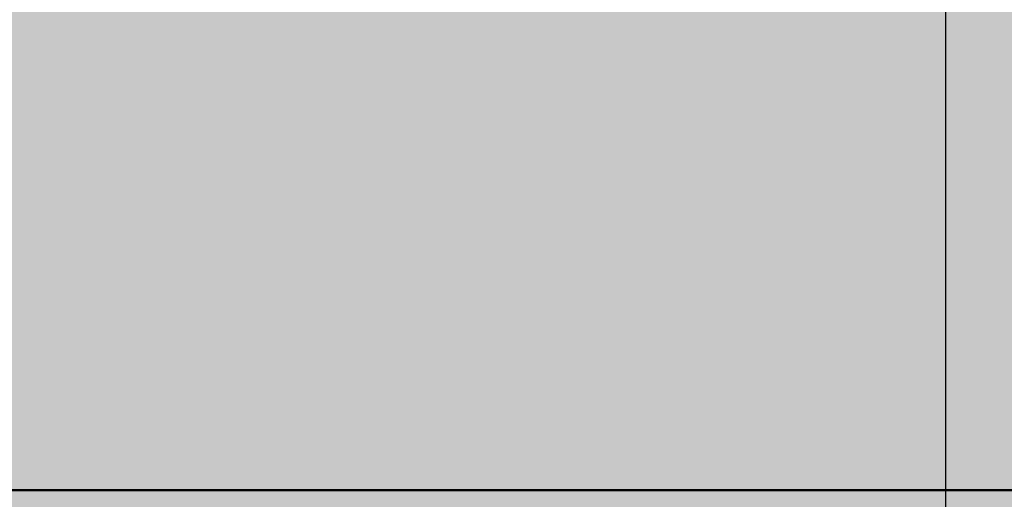
# Model space of a CAD drawing. Units: millimetres. Extents: x 0 to 2267, y 0 to 1823.
# Tile 149 of 256: x 1833.61 to 1844.05, y 1117.32 to 1122.41. Entities that reach past the tile are written whole.
import ezdxf

# ---------------------------------------------------------------- set-up
doc = ezdxf.new("R2010")
doc.units = ezdxf.units.MM
doc.header["$MEASUREMENT"] = 0
for name, color, linetype, lineweight in [('M-DIMS', 2, 'Continuous', 25), ('M-HATC', 252, 'Continuous', 18), ('M-OUTL', 7, 'Continuous', 50)]:
    doc.layers.add(name, color=color, linetype=linetype, lineweight=lineweight)
doc.styles.get("Standard").update_dxf_attribs({"font": 'arial.ttf'})
doc.dimstyles.get("Standard").update_dxf_attribs({"dimtxt": 7, "dimasz": 4, "dimexe": 0.18, "dimexo": 0.0625, "dimgap": 0.09, "dimtad": 0, "dimdec": 0, "dimzin": 0, "dimdsep": 46, "dimtxsty": 'Standard', "dimcen": 0.09, "dimadec": 0, "dimazin": 0, "dimtfac": 1, "dimtdec": 0, "dimtofl": 0, "dimtmove": 0, "dimatfit": 3, "dimfxl": 1, "dimtolj": 1, "dimtzin": 0, "dimarcsym": 0})

# ---------------------------------------------------------------- blocks, each defined once
blk = doc.blocks.new('*D1')
at = {"layer": 'Defpoints', "color": 0, "transparency": 16777216}
for p in [(1593.429, 1127.417), (1843.429, 1127.417), (1843.429, 955.628)]:
    blk.add_point(p, dxfattribs=at)
at = {"layer": 'M-DIMS', "color": 0, "lineweight": -2, "transparency": 16777216}
for p, q in [((1593.429, 1127.355), (1593.429, 955.448)), ((1843.429, 1127.355), (1843.429, 955.448)), ((1597.429, 955.628), (1710.558, 955.628)), ((1839.429, 955.628), (1726.3, 955.628))]:
    blk.add_line(p, q, dxfattribs=at)
at = {"layer": 'M-DIMS', "color": 0, "transparency": 16777216}
for points in [[(1597.429, 956.294), (1597.429, 954.961), (1593.429, 955.628)], [(1839.429, 956.294), (1839.429, 954.961), (1843.429, 955.628)]]:
    blk.add_solid(points, dxfattribs=at)
at = {"layer": 'M-DIMS', "color": 0, "transparency": 16777216, "insert": (1718.429, 955.628), "char_height": 7, "attachment_point": 5}
blk.add_mtext('\\A1;250', dxfattribs=at)

msp = doc.modelspace()

# ---------------------------------------------------------------- hatches: boundary and pattern name
at = {"layer": 'M-HATC'}
h = msp.add_hatch(color=256, dxfattribs=at)
h.dxf.hatch_style = 1
h.paths.add_polyline_path([(2065.771, 1618.062, 0.236068), (2055.771, 1638.062), (1381.087, 1638.062, 0.236068), (1371.087, 1618.062), (1371.087, 1603.062), (2055.771, 1603.062), (2065.771, 1603.062)])
h.paths.add_polyline_path([(2062.772, 1550.296), (2062.772, 1560.296), (1374.086, 1560.296), (1374.086, 1550.296), (1374.086, 1540.296), (1384.086, 1540.296), (1389.086, 1540.296), (2062.772, 1540.296)])
h.paths.add_polyline_path([(1930.929, 1282.766), (1505.929, 1282.766), (1587.628, 1235.597, 0.131652), (1600.128, 1232.247), (1836.73, 1232.247, 0.131652), (1849.23, 1235.597)])
h.paths.add_polyline_path([(1930.929, 1117.417), (1905.929, 1117.417), (1505.929, 1117.417), (1505.929, 1077.417), (1930.929, 1077.417)])
h = msp.add_hatch(color=256, dxfattribs=at)
h.dxf.hatch_style = 1
h.paths.add_polyline_path([(2055.771, 1603.062), (1381.087, 1603.062), (1381.087, 1598.062), (2055.771, 1598.062)])
h.paths.add_polyline_path([(2055.771, 1598.062), (1381.087, 1598.062), (1381.087, 1593.062), (2055.771, 1593.062)])
h.paths.add_polyline_path([(2051.307, 1536.761), (1385.55, 1536.761), (1385.55, 1526.761), (1387.55, 1526.761), (1388.537, 1525.053), (1385.332, 1521.233), (1385.332, 1521.223), (2050.254, 1522.749), (2048.321, 1525.053), (2049.307, 1526.761), (2051.307, 1526.761)])
edge = h.paths.add_edge_path()
edge.add_arc((1847.535, 1379.149), 135, 222.60306, 222.89085, ccw=False)
edge.add_line((1748.166, 1287.766), (1683.092, 1287.766))
edge.add_arc((1583.724, 1379.149), 135, 317.10915, 317.39694, ccw=False)
edge.add_arc((1678.969, 1290.671), 5, 222.8909, 317.1091, ccw=False)
edge.add_arc((1774.213, 1379.149), 135, 222.60306, 222.89085, ccw=False)
edge.add_line((1674.845, 1287.766), (1609.771, 1287.766))
edge.add_arc((1510.403, 1379.149), 135, 317.10915, 317.39694, ccw=False)
edge.add_arc((1605.647, 1290.671), 5, 222.8909, 317.1091, ccw=False)
edge.add_arc((1700.892, 1379.149), 135, 222.60306, 222.89085, ccw=False)
edge.add_line((1601.524, 1287.766), (1536.45, 1287.766))
edge.add_arc((1437.081, 1379.149), 135, 317.10915, 317.39694, ccw=False)
edge.add_arc((1532.326, 1290.671), 5, 222.8909, 317.1091, ccw=False)
edge.add_arc((1627.571, 1379.149), 135, 222.60306, 222.89085, ccw=False)
edge.add_line((1528.203, 1287.766), (1505.929, 1287.766))
edge.add_spline(control_points=[(1505.929, 1287.766), (1504.262, 1287.766), (1504.262, 1282.766), (1505.929, 1282.766)], knot_values=[0, 0, 0, 0, 5, 5, 5, 5], degree=3, periodic=0)
edge.add_line((1505.929, 1282.766), (1930.929, 1282.766))
edge.add_spline(control_points=[(1930.929, 1282.766), (1932.596, 1282.766), (1932.596, 1287.766), (1930.929, 1287.766)], knot_values=[0, 0, 0, 0, 5, 5, 5, 5], degree=3, periodic=0)
edge.add_line((1930.929, 1287.766), (1903.056, 1287.766))
edge.add_arc((1803.688, 1379.149), 135, 317.10915, 317.39694, ccw=False)
edge.add_arc((1898.932, 1290.671), 5, 222.8909, 317.1091, ccw=False)
edge.add_arc((1994.177, 1379.149), 135, 222.60306, 222.89085, ccw=False)
edge.add_line((1894.809, 1287.766), (1829.735, 1287.766))
edge.add_arc((1730.366, 1379.149), 135, 317.10915, 317.39694, ccw=False)
edge.add_arc((1825.611, 1290.671), 5, 222.8909, 317.1091, ccw=False)
edge.add_arc((1920.856, 1379.149), 135, 222.60306, 222.89085, ccw=False)
edge.add_line((1821.487, 1287.766), (1756.413, 1287.766))
edge.add_arc((1657.045, 1379.149), 135, 317.10915, 317.39694, ccw=False)
edge.add_arc((1752.29, 1290.671), 5, 222.8909, 317.1091, ccw=False)
edge = h.paths.add_edge_path()
edge.add_spline(control_points=[(1843.429, 1227.247), (1845.096, 1227.247), (1845.096, 1232.247), (1843.429, 1232.247)], knot_values=[0, 0, 0, 0, 5, 5, 5, 5], degree=3, periodic=0)
edge.add_line((1843.429, 1232.247), (1593.429, 1232.247))
edge.add_spline(control_points=[(1593.429, 1232.247), (1591.762, 1232.247), (1591.762, 1227.247), (1593.429, 1227.247)], knot_values=[0, 0, 0, 0, 5, 5, 5, 5], degree=3, periodic=0)
edge.add_line((1593.429, 1227.247), (1843.429, 1227.247))
h.paths.add_polyline_path([(1905.929, 1127.417), (1530.929, 1127.417, 0.414214), (1520.929, 1117.417), (1530.929, 1117.417), (1915.929, 1117.417, 0.414214)])
edge = h.paths.add_edge_path()
edge.add_arc((1397.086, 1498.408), 12.73, 90.7821, 190.8787, ccw=False)
edge.add_line((1396.912, 1511.136), (1428.01, 1511.349))
edge.add_line((1428.01, 1511.349), (1433.01, 1511.349))
edge.add_line((1433.01, 1511.349), (1434.439, 1511.349))
edge.add_arc((1419.474, 1498.08), 20, 41.561, 74.0821)
edge.add_line((1424.959, 1517.314), (1399.935, 1517.256))
edge.add_spline(control_points=[(1399.931, 1517.256), (1399.884, 1517.213), (1399.833, 1517.169), (1399.777, 1517.124)], knot_values=[11.567499, 11.567499, 11.567499, 11.567499, 11.814249, 11.814249, 11.814249, 11.814249], degree=3, periodic=0)
edge.add_spline(control_points=[(1399.633, 1517.01), (1399.583, 1516.972), (1399.531, 1516.934), (1399.476, 1516.895)], knot_values=[11.167718, 11.167718, 11.167718, 11.167718, 11.365188, 11.365188, 11.365188, 11.365188], degree=3, periodic=0)
edge.add_spline(control_points=[(1399.34, 1516.8), (1399.151, 1516.672), (1398.938, 1516.538), (1398.704, 1516.399)], knot_values=[10.376405, 10.376405, 10.376405, 10.376405, 11.00994, 11.00994, 11.00994, 11.00994], degree=3, periodic=0)
edge.add_spline(control_points=[(1398.657, 1516.372), (1398.579, 1516.326), (1398.498, 1516.28), (1398.415, 1516.233)], knot_values=[10.125175, 10.125175, 10.125175, 10.125175, 10.334406, 10.334406, 10.334406, 10.334406], degree=3, periodic=0)
edge.add_spline(control_points=[(1398.264, 1516.149), (1398.196, 1516.111), (1398.126, 1516.073), (1398.055, 1516.035)], knot_values=[9.832246, 9.832246, 9.832246, 9.832246, 9.999658, 9.999658, 9.999658, 9.999658], degree=3, periodic=0)
edge.add_spline(control_points=[(1397.999, 1516.005), (1397.731, 1515.862), (1397.446, 1515.717), (1397.147, 1515.571)], knot_values=[9.161808, 9.161808, 9.161808, 9.161808, 9.787769, 9.787769, 9.787769, 9.787769], degree=3, periodic=0)
edge.add_spline(control_points=[(1397.147, 1515.571), (1396.842, 1515.423), (1396.522, 1515.274), (1396.191, 1515.126)], knot_values=[8.524455, 8.524455, 8.524455, 8.524455, 9.161808, 9.161808, 9.161808, 9.161808], degree=3, periodic=0)
edge.add_spline(control_points=[(1396.078, 1515.076), (1395.985, 1515.035), (1395.892, 1514.994), (1395.798, 1514.953)], knot_values=[8.275193, 8.275193, 8.275193, 8.275193, 8.451726, 8.451726, 8.451726, 8.451726], degree=3, periodic=0)
edge.add_spline(control_points=[(1395.602, 1514.869), (1395.5, 1514.826), (1395.397, 1514.782), (1395.293, 1514.739)], knot_values=[7.962917, 7.962917, 7.962917, 7.962917, 8.152764, 8.152764, 8.152764, 8.152764], degree=3, periodic=0)
edge.add_spline(control_points=[(1395.212, 1514.706), (1394.828, 1514.547), (1394.435, 1514.393), (1394.036, 1514.244)], knot_values=[7.21254, 7.21254, 7.21254, 7.21254, 7.913148, 7.913148, 7.913148, 7.913148], degree=3, periodic=0)
edge.add_spline(control_points=[(1394.036, 1514.244), (1393.708, 1514.121), (1393.375, 1514.003), (1393.043, 1513.889)], knot_values=[6.633733, 6.633733, 6.633733, 6.633733, 7.21254, 7.21254, 7.21254, 7.21254], degree=3, periodic=0)
edge.add_spline(control_points=[(1392.821, 1513.815), (1392.72, 1513.781), (1392.618, 1513.748), (1392.517, 1513.715)], knot_values=[6.328796, 6.328796, 6.328796, 6.328796, 6.505493, 6.505493, 6.505493, 6.505493], degree=3, periodic=0)
edge.add_spline(control_points=[(1392.517, 1513.715), (1392.319, 1513.652), (1392.121, 1513.59), (1391.924, 1513.531)], knot_values=[5.984605, 5.984605, 5.984605, 5.984605, 6.328796, 6.328796, 6.328796, 6.328796], degree=3, periodic=0)
edge.add_spline(control_points=[(1391.792, 1513.491), (1391.312, 1513.35), (1390.838, 1513.224), (1390.378, 1513.117)], knot_values=[5.066697, 5.066697, 5.066697, 5.066697, 5.907055, 5.907055, 5.907055, 5.907055], degree=3, periodic=0)
edge.add_spline(control_points=[(1390.378, 1513.117), (1390.18, 1513.071), (1389.984, 1513.028), (1389.791, 1512.99)], knot_values=[4.70367, 4.70367, 4.70367, 4.70367, 5.066695, 5.066695, 5.066695, 5.066695], degree=3, periodic=0)
edge.add_spline(control_points=[(1389.422, 1512.92), (1389.246, 1512.889), (1389.073, 1512.862), (1388.904, 1512.838)], knot_values=[4.130571, 4.130571, 4.130571, 4.130571, 4.469816, 4.469816, 4.469816, 4.469816], degree=3, periodic=0)
edge.add_spline(control_points=[(1388.904, 1512.838), (1388.591, 1512.795), (1388.291, 1512.764), (1388.007, 1512.749)], knot_values=[3.504031, 3.504031, 3.504031, 3.504031, 4.130571, 4.130571, 4.130571, 4.130571], degree=3, periodic=0)
edge.add_spline(control_points=[(1387.936, 1512.746), (1387.854, 1512.742), (1387.773, 1512.74), (1387.694, 1512.739)], knot_values=[3.268866, 3.268866, 3.268866, 3.268866, 3.451164, 3.451164, 3.451164, 3.451164], degree=3, periodic=0)
edge.add_spline(control_points=[(1387.335, 1512.744), (1387.208, 1512.75), (1387.085, 1512.76), (1386.967, 1512.774)], knot_values=[2.670686, 2.670686, 2.670686, 2.670686, 2.984, 2.984, 2.984, 2.984], degree=3, periodic=0)
edge.add_spline(control_points=[(1386.833, 1512.792), (1386.821, 1512.794), (1386.809, 1512.796), (1386.797, 1512.798)], knot_values=[2.516981, 2.516981, 2.516981, 2.516981, 2.549528, 2.549528, 2.549528, 2.549528], degree=3, periodic=0)
edge.add_spline(control_points=[(1386.453, 1512.873), (1386.426, 1512.881), (1386.399, 1512.889), (1386.373, 1512.897)], knot_values=[2.095869, 2.095869, 2.095869, 2.095869, 2.17941, 2.17941, 2.17941, 2.17941], degree=3, periodic=0)
edge.add_spline(control_points=[(1386.069, 1513.019), (1386.063, 1513.022), (1386.058, 1513.025), (1386.052, 1513.028)], knot_values=[1.72453, 1.72453, 1.72453, 1.72453, 1.745933, 1.745933, 1.745933, 1.745933], degree=3, periodic=0)
edge.add_arc((1399.474, 1498.08), 20, 131.8243, 180)
edge.add_arc((1630.334, 1505.548), 250.971, 181.70518, 236.42798)
edge.add_arc((1605.34, 1483.304), 218.782, 238.66083, 243.34961)
edge.add_arc((1647.091, 1510.359), 262.899, 183.12984, 237.85344, ccw=False)
h.paths.add_polyline_path([(1406.537, 1391.964, 0.149382), (1491.551, 1296.442, -0.129517)], flags=17)
edge = h.paths.add_edge_path()
edge.add_arc((2037.384, 1498.08), 20, 0, 48.2659)
edge.add_spline(control_points=[(2050.697, 1513.005), (2050.651, 1512.985), (2050.603, 1512.966), (2050.554, 1512.948)], knot_values=[1.835652, 1.835652, 1.835652, 1.835652, 2.000781, 2.000781, 2.000781, 2.000781], degree=3, periodic=0)
edge.add_spline(control_points=[(2050.462, 1512.917), (2050.479, 1512.922), (2050.496, 1512.928), (2050.513, 1512.934)], knot_values=[2.045477, 2.045477, 2.045477, 2.045477, 2.101389, 2.101389, 2.101389, 2.101389], degree=3, periodic=0)
edge.add_spline(control_points=[(2050.129, 1512.834), (2050.198, 1512.847), (2050.266, 1512.862), (2050.331, 1512.879)], knot_values=[2.237629, 2.237629, 2.237629, 2.237629, 2.435841, 2.435841, 2.435841, 2.435841], degree=3, periodic=0)
edge.add_spline(control_points=[(2050.095, 1512.828), (2050.106, 1512.83), (2050.118, 1512.832), (2050.129, 1512.834)], knot_values=[2.435841, 2.435841, 2.435841, 2.435841, 2.468321, 2.468321, 2.468321, 2.468321], degree=3, periodic=0)
edge.add_spline(control_points=[(2049.784, 1512.785), (2049.855, 1512.792), (2049.924, 1512.801), (2049.992, 1512.811)], knot_values=[2.563852, 2.563852, 2.563852, 2.563852, 2.748541, 2.748541, 2.748541, 2.748541], degree=3, periodic=0)
edge.add_spline(control_points=[(2049.405, 1512.762), (2049.536, 1512.765), (2049.663, 1512.773), (2049.784, 1512.785)], knot_values=[2.748541, 2.748541, 2.748541, 2.748541, 3.064882, 3.064882, 3.064882, 3.064882], degree=3, periodic=0)
edge.add_spline(control_points=[(2049.17, 1512.76), (2049.234, 1512.759), (2049.297, 1512.759), (2049.358, 1512.761)], knot_values=[3.102309, 3.102309, 3.102309, 3.102309, 3.2503, 3.2503, 3.2503, 3.2503], degree=3, periodic=0)
edge.add_spline(control_points=[(2048.857, 1512.769), (2048.964, 1512.764), (2049.068, 1512.761), (2049.17, 1512.76)], knot_values=[3.2503, 3.2503, 3.2503, 3.2503, 3.486069, 3.486069, 3.486069, 3.486069], degree=3, periodic=0)
edge.add_spline(control_points=[(2048.692, 1512.779), (2048.373, 1512.801), (2048.035, 1512.841), (2047.682, 1512.897)], knot_values=[3.606429, 3.606429, 3.606429, 3.606429, 4.2989, 4.2989, 4.2989, 4.2989], degree=3, periodic=0)
edge.add_spline(control_points=[(2047.682, 1512.897), (2047.546, 1512.919), (2047.408, 1512.942), (2047.268, 1512.969)], knot_values=[4.2989, 4.2989, 4.2989, 4.2989, 4.565769, 4.565769, 4.565769, 4.565769], degree=3, periodic=0)
edge.add_spline(control_points=[(2047.268, 1512.969), (2047.145, 1512.991), (2047.021, 1513.016), (2046.895, 1513.042)], knot_values=[4.565769, 4.565769, 4.565769, 4.565769, 4.799971, 4.799971, 4.799971, 4.799971], degree=3, periodic=0)
edge.add_spline(control_points=[(2046.895, 1513.042), (2046.529, 1513.119), (2046.151, 1513.209), (2045.768, 1513.311)], knot_values=[4.799971, 4.799971, 4.799971, 4.799971, 5.483718, 5.483718, 5.483718, 5.483718], degree=3, periodic=0)
edge.add_spline(control_points=[(2045.768, 1513.311), (2045.372, 1513.415), (2044.97, 1513.532), (2044.566, 1513.659)], knot_values=[5.483718, 5.483718, 5.483718, 5.483718, 6.187866, 6.187866, 6.187866, 6.187866], degree=3, periodic=0)
edge.add_spline(control_points=[(2044.566, 1513.659), (2044.415, 1513.706), (2044.263, 1513.755), (2044.112, 1513.805)], knot_values=[6.187866, 6.187866, 6.187866, 6.187866, 6.451551, 6.451551, 6.451551, 6.451551], degree=3, periodic=0)
edge.add_spline(control_points=[(2044.112, 1513.805), (2043.997, 1513.843), (2043.882, 1513.881), (2043.767, 1513.92)], knot_values=[6.451551, 6.451551, 6.451551, 6.451551, 6.651434, 6.651434, 6.651434, 6.651434], degree=3, periodic=0)
edge.add_spline(control_points=[(2043.767, 1513.92), (2043.372, 1514.055), (2042.977, 1514.198), (2042.589, 1514.346)], knot_values=[6.651434, 6.651434, 6.651434, 6.651434, 7.338879, 7.338879, 7.338879, 7.338879], degree=3, periodic=0)
edge.add_spline(control_points=[(2042.589, 1514.346), (2042.164, 1514.507), (2041.746, 1514.675), (2041.341, 1514.846)], knot_values=[7.338879, 7.338879, 7.338879, 7.338879, 8.089209, 8.089209, 8.089209, 8.089209], degree=3, periodic=0)
edge.add_spline(control_points=[(2041.341, 1514.846), (2041.103, 1514.946), (2040.869, 1515.048), (2040.64, 1515.15)], knot_values=[8.089209, 8.089209, 8.089209, 8.089209, 8.529587, 8.529587, 8.529587, 8.529587], degree=3, periodic=0)
edge.add_spline(control_points=[(2040.51, 1515.209), (2040.082, 1515.402), (2039.675, 1515.597), (2039.295, 1515.789)], knot_values=[8.613818, 8.613818, 8.613818, 8.613818, 9.44571, 9.44571, 9.44571, 9.44571], degree=3, periodic=0)
edge.add_spline(control_points=[(2039.295, 1515.789), (2039.062, 1515.907), (2038.839, 1516.025), (2038.629, 1516.14)], knot_values=[9.44571, 9.44571, 9.44571, 9.44571, 9.956404, 9.956404, 9.956404, 9.956404], degree=3, periodic=0)
edge.add_spline(control_points=[(2038.629, 1516.14), (2038.519, 1516.2), (2038.412, 1516.26), (2038.309, 1516.319)], knot_values=[9.956404, 9.956404, 9.956404, 9.956404, 10.223542, 10.223542, 10.223542, 10.223542], degree=3, periodic=0)
edge.add_spline(control_points=[(2038.309, 1516.319), (2038.214, 1516.374), (2038.122, 1516.428), (2038.033, 1516.481)], knot_values=[10.223542, 10.223542, 10.223542, 10.223542, 10.47051, 10.47051, 10.47051, 10.47051], degree=3, periodic=0)
edge.add_spline(control_points=[(2038.033, 1516.481), (2037.786, 1516.63), (2037.564, 1516.773), (2037.372, 1516.909)], knot_values=[10.47051, 10.47051, 10.47051, 10.47051, 11.15767, 11.15767, 11.15767, 11.15767], degree=3, periodic=0)
edge.add_spline(control_points=[(2037.372, 1516.909), (2037.279, 1516.975), (2037.193, 1517.04), (2037.114, 1517.102)], knot_values=[11.15767, 11.15767, 11.15767, 11.15767, 11.49227, 11.49227, 11.49227, 11.49227], degree=3, periodic=0)
edge.add_spline(control_points=[(2036.856, 1517.326), (2036.915, 1517.269), (2036.981, 1517.21), (2037.056, 1517.149)], knot_values=[11.577341, 11.577341, 11.577341, 11.577341, 11.91035, 11.91035, 11.91035, 11.91035], degree=3, periodic=0)
edge.add_spline(control_points=[(2036.807, 1517.375), (2036.823, 1517.359), (2036.839, 1517.342), (2036.856, 1517.326)], knot_values=[11.91035, 11.91035, 11.91035, 11.91035, 12.007402, 12.007402, 12.007402, 12.007402], degree=3, periodic=0)
edge.add_spline(control_points=[(2036.702, 1517.494), (2036.71, 1517.483), (2036.72, 1517.472), (2036.729, 1517.461)], knot_values=[12.184155, 12.184155, 12.184155, 12.184155, 12.255409, 12.255409, 12.255409, 12.255409], degree=3, periodic=0)
edge.add_spline(control_points=[(2036.616, 1517.621), (2036.62, 1517.613), (2036.624, 1517.606), (2036.629, 1517.598)], knot_values=[12.487913, 12.487913, 12.487913, 12.487913, 12.541035, 12.541035, 12.541035, 12.541035], degree=3, periodic=0)
edge.add_spline(control_points=[(2036.563, 1517.786), (2036.564, 1517.779), (2036.564, 1517.773), (2036.565, 1517.766)], knot_values=[12.911761, 12.911761, 12.911761, 12.911761, 12.968286, 12.968286, 12.968286, 12.968286], degree=3, periodic=0)
edge.add_spline(control_points=[(2036.617, 1517.93), (2036.612, 1517.926), (2036.609, 1517.921), (2036.605, 1517.916)], knot_values=[13.382527, 13.382527, 13.382527, 13.382527, 13.433791, 13.433791, 13.433791, 13.433791], degree=3, periodic=0)
edge.add_spline(control_points=[(2036.749, 1518.017), (2036.736, 1518.012), (2036.724, 1518.006), (2036.712, 1518)], knot_values=[13.726299, 13.726299, 13.726299, 13.726299, 13.809928, 13.809928, 13.809928, 13.809928], degree=3, periodic=0)
edge.add_spline(control_points=[(2036.86, 1518.053), (2036.839, 1518.047), (2036.818, 1518.042), (2036.799, 1518.035)], knot_values=[13.910887, 13.910887, 13.910887, 13.910887, 14.02153, 14.02153, 14.02153, 14.02153], degree=3, periodic=0)
edge.add_line((2036.964, 1518.08), (2032.384, 1518.08))
edge.add_line((2032.384, 1518.08), (2027.384, 1518.08))
edge.add_line((2027.384, 1518.08), (2022.384, 1518.08))
edge.add_line((2022.384, 1518.08), (2017.384, 1518.08))
edge.add_arc((2017.384, 1498.08), 20, 90, 138.439)
edge.add_line((2002.419, 1511.349), (2003.848, 1511.349))
edge.add_line((2003.848, 1511.349), (2008.848, 1511.349))
edge.add_line((2008.848, 1511.349), (2039.772, 1511.138))
edge.add_arc((2039.772, 1498.408), 12.73, -10.8787, 90, ccw=False)
edge.add_arc((1789.767, 1510.359), 262.899, 302.14656, 356.87016, ccw=False)
edge.add_arc((1831.518, 1483.304), 218.782, 296.65039, 301.33917)
edge.add_arc((1806.524, 1505.548), 250.971, 303.57202, 358.29482)
h.paths.add_polyline_path([(2030.321, 1391.964, -0.129517), (1945.307, 1296.442, 0.149382)], flags=17)
edge = h.paths.add_edge_path()
edge.add_spline(control_points=[(2037.246, 1518.082), (2037.29, 1518.081), (2037.336, 1518.08), (2037.384, 1518.08)], knot_values=[0.000012, 0.000012, 0.000012, 0.000012, 0.144754, 0.144754, 0.144754, 0.144754], degree=3, periodic=0)
edge.add_line((2037.336, 1518.08), (2037.01, 1518.08))
edge.add_spline(control_points=[(2037.01, 1518.08), (2036.982, 1518.077), (2036.956, 1518.073), (2036.931, 1518.068)], knot_values=[14.13465, 14.13465, 14.13465, 14.13465, 14.247197, 14.247197, 14.247197, 14.247197], degree=3, periodic=0)
edge.add_spline(control_points=[(2036.931, 1518.068), (2036.928, 1518.067), (2036.924, 1518.067), (2036.921, 1518.066)], knot_values=[14.118315, 14.118315, 14.118315, 14.118315, 14.13465, 14.13465, 14.13465, 14.13465], degree=3, periodic=0)
edge.add_spline(control_points=[(2036.921, 1518.066), (2036.912, 1518.064), (2036.903, 1518.063), (2036.895, 1518.061)], knot_values=[14.078086, 14.078086, 14.078086, 14.078086, 14.118315, 14.118315, 14.118315, 14.118315], degree=3, periodic=0)
edge.add_spline(control_points=[(2036.895, 1518.061), (2036.883, 1518.058), (2036.872, 1518.056), (2036.86, 1518.053)], knot_values=[14.02153, 14.02153, 14.02153, 14.02153, 14.078086, 14.078086, 14.078086, 14.078086], degree=3, periodic=0)
edge.add_spline(control_points=[(2036.86, 1518.053), (2036.839, 1518.047), (2036.818, 1518.042), (2036.799, 1518.035)], knot_values=[13.910887, 13.910887, 13.910887, 13.910887, 14.02153, 14.02153, 14.02153, 14.02153], degree=3, periodic=0)
edge.add_spline(control_points=[(2036.799, 1518.035), (2036.798, 1518.035), (2036.797, 1518.035), (2036.797, 1518.035)], knot_values=[13.906906, 13.906906, 13.906906, 13.906906, 13.910887, 13.910887, 13.910887, 13.910887], degree=3, periodic=0)
edge.add_spline(control_points=[(2036.797, 1518.035), (2036.788, 1518.032), (2036.78, 1518.029), (2036.772, 1518.026)], knot_values=[13.857826, 13.857826, 13.857826, 13.857826, 13.906906, 13.906906, 13.906906, 13.906906], degree=3, periodic=0)
edge.add_spline(control_points=[(2036.772, 1518.026), (2036.764, 1518.023), (2036.756, 1518.02), (2036.749, 1518.017)], knot_values=[13.809928, 13.809928, 13.809928, 13.809928, 13.857826, 13.857826, 13.857826, 13.857826], degree=3, periodic=0)
edge.add_spline(control_points=[(2036.749, 1518.017), (2036.736, 1518.012), (2036.724, 1518.006), (2036.712, 1518)], knot_values=[13.726299, 13.726299, 13.726299, 13.726299, 13.809928, 13.809928, 13.809928, 13.809928], degree=3, periodic=0)
edge.add_spline(control_points=[(2036.712, 1518), (2036.712, 1518), (2036.712, 1518), (2036.711, 1518)], knot_values=[13.723993, 13.723993, 13.723993, 13.723993, 13.726299, 13.726299, 13.726299, 13.726299], degree=3, periodic=0)
edge.add_spline(control_points=[(2036.711, 1518), (2036.706, 1517.997), (2036.701, 1517.994), (2036.696, 1517.992)], knot_values=[13.686536, 13.686536, 13.686536, 13.686536, 13.723993, 13.723993, 13.723993, 13.723993], degree=3, periodic=0)
edge.add_spline(control_points=[(2036.696, 1517.992), (2036.692, 1517.989), (2036.687, 1517.987), (2036.683, 1517.984)], knot_values=[13.651251, 13.651251, 13.651251, 13.651251, 13.686536, 13.686536, 13.686536, 13.686536], degree=3, periodic=0)
edge.add_spline(control_points=[(2036.683, 1517.984), (2036.676, 1517.98), (2036.67, 1517.976), (2036.664, 1517.971)], knot_values=[13.596804, 13.596804, 13.596804, 13.596804, 13.651251, 13.651251, 13.651251, 13.651251], degree=3, periodic=0)
edge.add_spline(control_points=[(2036.664, 1517.971), (2036.664, 1517.971), (2036.663, 1517.971), (2036.663, 1517.971)], knot_values=[13.593956, 13.593956, 13.593956, 13.593956, 13.596804, 13.596804, 13.596804, 13.596804], degree=3, periodic=0)
edge.add_spline(control_points=[(2036.663, 1517.971), (2036.66, 1517.969), (2036.658, 1517.967), (2036.655, 1517.965)], knot_values=[13.570322, 13.570322, 13.570322, 13.570322, 13.593956, 13.593956, 13.593956, 13.593956], degree=3, periodic=0)
edge.add_spline(control_points=[(2036.655, 1517.965), (2036.653, 1517.963), (2036.65, 1517.961), (2036.647, 1517.959)], knot_values=[13.545477, 13.545477, 13.545477, 13.545477, 13.570322, 13.570322, 13.570322, 13.570322], degree=3, periodic=0)
edge.add_spline(control_points=[(2036.647, 1517.959), (2036.647, 1517.959), (2036.647, 1517.959), (2036.647, 1517.959)], knot_values=[13.543931, 13.543931, 13.543931, 13.543931, 13.545477, 13.545477, 13.545477, 13.545477], degree=3, periodic=0)
edge.add_spline(control_points=[(2036.647, 1517.959), (2036.641, 1517.954), (2036.636, 1517.949), (2036.631, 1517.945)], knot_values=[13.488237, 13.488237, 13.488237, 13.488237, 13.543931, 13.543931, 13.543931, 13.543931], degree=3, periodic=0)
edge.add_spline(control_points=[(2036.631, 1517.945), (2036.628, 1517.942), (2036.626, 1517.94), (2036.623, 1517.937)], knot_values=[13.460307, 13.460307, 13.460307, 13.460307, 13.488237, 13.488237, 13.488237, 13.488237], degree=3, periodic=0)
edge.add_spline(control_points=[(2036.623, 1517.937), (2036.622, 1517.936), (2036.62, 1517.934), (2036.618, 1517.932)], knot_values=[13.439712, 13.439712, 13.439712, 13.439712, 13.460307, 13.460307, 13.460307, 13.460307], degree=3, periodic=0)
edge.add_spline(control_points=[(2036.618, 1517.932), (2036.618, 1517.931), (2036.617, 1517.931), (2036.617, 1517.93)], knot_values=[13.433791, 13.433791, 13.433791, 13.433791, 13.439712, 13.439712, 13.439712, 13.439712], degree=3, periodic=0)
edge.add_spline(control_points=[(2036.617, 1517.93), (2036.612, 1517.926), (2036.609, 1517.921), (2036.605, 1517.916)], knot_values=[13.382527, 13.382527, 13.382527, 13.382527, 13.433791, 13.433791, 13.433791, 13.433791], degree=3, periodic=0)
edge.add_spline(control_points=[(2036.605, 1517.916), (2036.603, 1517.913), (2036.6, 1517.91), (2036.598, 1517.907)], knot_values=[13.350017, 13.350017, 13.350017, 13.350017, 13.382527, 13.382527, 13.382527, 13.382527], degree=3, periodic=0)
edge.add_spline(control_points=[(2036.598, 1517.907), (2036.597, 1517.906), (2036.596, 1517.904), (2036.595, 1517.903)], knot_values=[13.333922, 13.333922, 13.333922, 13.333922, 13.350017, 13.350017, 13.350017, 13.350017], degree=3, periodic=0)
edge.add_spline(control_points=[(2036.595, 1517.903), (2036.595, 1517.902), (2036.594, 1517.901), (2036.593, 1517.9)], knot_values=[13.323828, 13.323828, 13.323828, 13.323828, 13.333922, 13.333922, 13.333922, 13.333922], degree=3, periodic=0)
edge.add_spline(control_points=[(2036.593, 1517.9), (2036.59, 1517.895), (2036.588, 1517.891), (2036.585, 1517.886)], knot_values=[13.277545, 13.277545, 13.277545, 13.277545, 13.323828, 13.323828, 13.323828, 13.323828], degree=3, periodic=0)
edge.add_spline(control_points=[(2036.585, 1517.886), (2036.584, 1517.883), (2036.582, 1517.879), (2036.58, 1517.875)], knot_values=[13.240119, 13.240119, 13.240119, 13.240119, 13.277545, 13.277545, 13.277545, 13.277545], degree=3, periodic=0)
edge.add_spline(control_points=[(2036.58, 1517.875), (2036.58, 1517.874), (2036.579, 1517.873), (2036.578, 1517.872)], knot_values=[13.228211, 13.228211, 13.228211, 13.228211, 13.240119, 13.240119, 13.240119, 13.240119], degree=3, periodic=0)
edge.add_spline(control_points=[(2036.578, 1517.872), (2036.578, 1517.87), (2036.577, 1517.869), (2036.577, 1517.868)], knot_values=[13.215717, 13.215717, 13.215717, 13.215717, 13.228211, 13.228211, 13.228211, 13.228211], degree=3, periodic=0)
edge.add_spline(control_points=[(2036.577, 1517.868), (2036.575, 1517.864), (2036.574, 1517.86), (2036.573, 1517.857)], knot_values=[13.179847, 13.179847, 13.179847, 13.179847, 13.215717, 13.215717, 13.215717, 13.215717], degree=3, periodic=0)
edge.add_spline(control_points=[(2036.573, 1517.857), (2036.571, 1517.851), (2036.57, 1517.846), (2036.569, 1517.841)], knot_values=[13.132017, 13.132017, 13.132017, 13.132017, 13.179847, 13.179847, 13.179847, 13.179847], degree=3, periodic=0)
edge.add_spline(control_points=[(2036.569, 1517.841), (2036.568, 1517.84), (2036.568, 1517.839), (2036.568, 1517.838)], knot_values=[13.122482, 13.122482, 13.122482, 13.122482, 13.132017, 13.132017, 13.132017, 13.132017], degree=3, periodic=0)
edge.add_spline(control_points=[(2036.568, 1517.838), (2036.568, 1517.836), (2036.567, 1517.835), (2036.567, 1517.833)], knot_values=[13.105592, 13.105592, 13.105592, 13.105592, 13.122482, 13.122482, 13.122482, 13.122482], degree=3, periodic=0)
edge.add_spline(control_points=[(2036.567, 1517.833), (2036.566, 1517.829), (2036.566, 1517.826), (2036.565, 1517.822)], knot_values=[13.074063, 13.074063, 13.074063, 13.074063, 13.105592, 13.105592, 13.105592, 13.105592], degree=3, periodic=0)
edge.add_spline(control_points=[(2036.565, 1517.822), (2036.565, 1517.822), (2036.565, 1517.822), (2036.565, 1517.822)], knot_values=[13.074043, 13.074043, 13.074043, 13.074043, 13.074063, 13.074063, 13.074063, 13.074063], degree=3, periodic=0)
edge.add_spline(control_points=[(2036.565, 1517.822), (2036.564, 1517.816), (2036.564, 1517.811), (2036.564, 1517.805)], knot_values=[13.021884, 13.021884, 13.021884, 13.021884, 13.074043, 13.074043, 13.074043, 13.074043], degree=3, periodic=0)
edge.add_spline(control_points=[(2036.564, 1517.805), (2036.564, 1517.804), (2036.564, 1517.803), (2036.564, 1517.803)], knot_values=[13.01674, 13.01674, 13.01674, 13.01674, 13.021884, 13.021884, 13.021884, 13.021884], degree=3, periodic=0)
edge.add_spline(control_points=[(2036.564, 1517.803), (2036.563, 1517.801), (2036.563, 1517.798), (2036.563, 1517.796)], knot_values=[12.996438, 12.996438, 12.996438, 12.996438, 13.01674, 13.01674, 13.01674, 13.01674], degree=3, periodic=0)
edge.add_spline(control_points=[(2036.563, 1517.796), (2036.563, 1517.793), (2036.563, 1517.789), (2036.563, 1517.786)], knot_values=[12.968286, 12.968286, 12.968286, 12.968286, 12.996438, 12.996438, 12.996438, 12.996438], degree=3, periodic=0)
edge.add_spline(control_points=[(2036.563, 1517.786), (2036.564, 1517.779), (2036.564, 1517.773), (2036.565, 1517.766)], knot_values=[12.911761, 12.911761, 12.911761, 12.911761, 12.968286, 12.968286, 12.968286, 12.968286], degree=3, periodic=0)
edge.add_spline(control_points=[(2036.565, 1517.766), (2036.565, 1517.766), (2036.565, 1517.766), (2036.565, 1517.766)], knot_values=[12.911017, 12.911017, 12.911017, 12.911017, 12.911761, 12.911761, 12.911761, 12.911761], degree=3, periodic=0)
edge.add_spline(control_points=[(2036.565, 1517.766), (2036.565, 1517.762), (2036.566, 1517.759), (2036.566, 1517.756)], knot_values=[12.88528, 12.88528, 12.88528, 12.88528, 12.911017, 12.911017, 12.911017, 12.911017], degree=3, periodic=0)
edge.add_spline(control_points=[(2036.566, 1517.756), (2036.567, 1517.753), (2036.567, 1517.751), (2036.568, 1517.748)], knot_values=[12.862519, 12.862519, 12.862519, 12.862519, 12.88528, 12.88528, 12.88528, 12.88528], degree=3, periodic=0)
edge.add_spline(control_points=[(2036.568, 1517.748), (2036.568, 1517.747), (2036.568, 1517.747), (2036.568, 1517.746)], knot_values=[12.858885, 12.858885, 12.858885, 12.858885, 12.862519, 12.862519, 12.862519, 12.862519], degree=3, periodic=0)
edge.add_spline(control_points=[(2036.568, 1517.746), (2036.569, 1517.74), (2036.571, 1517.733), (2036.572, 1517.726)], knot_values=[12.8053, 12.8053, 12.8053, 12.8053, 12.858885, 12.858885, 12.858885, 12.858885], degree=3, periodic=0)
edge.add_spline(control_points=[(2036.572, 1517.726), (2036.573, 1517.723), (2036.574, 1517.719), (2036.576, 1517.715)], knot_values=[12.775176, 12.775176, 12.775176, 12.775176, 12.8053, 12.8053, 12.8053, 12.8053], degree=3, periodic=0)
edge.add_spline(control_points=[(2036.576, 1517.715), (2036.576, 1517.713), (2036.577, 1517.71), (2036.578, 1517.708)], knot_values=[12.756759, 12.756759, 12.756759, 12.756759, 12.775176, 12.775176, 12.775176, 12.775176], degree=3, periodic=0)
edge.add_spline(control_points=[(2036.578, 1517.708), (2036.578, 1517.707), (2036.578, 1517.706), (2036.579, 1517.705)], knot_values=[12.748742, 12.748742, 12.748742, 12.748742, 12.756759, 12.756759, 12.756759, 12.756759], degree=3, periodic=0)
edge.add_spline(control_points=[(2036.579, 1517.705), (2036.581, 1517.698), (2036.583, 1517.692), (2036.586, 1517.685)], knot_values=[12.69959, 12.69959, 12.69959, 12.69959, 12.748742, 12.748742, 12.748742, 12.748742], degree=3, periodic=0)
edge.add_spline(control_points=[(2036.586, 1517.685), (2036.588, 1517.68), (2036.59, 1517.675), (2036.592, 1517.669)], knot_values=[12.659038, 12.659038, 12.659038, 12.659038, 12.69959, 12.69959, 12.69959, 12.69959], degree=3, periodic=0)
edge.add_spline(control_points=[(2036.592, 1517.669), (2036.594, 1517.665), (2036.596, 1517.66), (2036.598, 1517.656)], knot_values=[12.626806, 12.626806, 12.626806, 12.626806, 12.659038, 12.659038, 12.659038, 12.659038], degree=3, periodic=0)
edge.add_spline(control_points=[(2036.598, 1517.656), (2036.598, 1517.655), (2036.599, 1517.654), (2036.599, 1517.653)], knot_values=[12.619394, 12.619394, 12.619394, 12.619394, 12.626806, 12.626806, 12.626806, 12.626806], degree=3, periodic=0)
edge.add_spline(control_points=[(2036.599, 1517.653), (2036.604, 1517.642), (2036.61, 1517.632), (2036.616, 1517.621)], knot_values=[12.541039, 12.541039, 12.541039, 12.541039, 12.619394, 12.619394, 12.619394, 12.619394], degree=3, periodic=0)
edge.add_spline(control_points=[(2036.616, 1517.621), (2036.616, 1517.621), (2036.616, 1517.621), (2036.616, 1517.621)], knot_values=[12.541035, 12.541035, 12.541035, 12.541035, 12.541039, 12.541039, 12.541039, 12.541039], degree=3, periodic=0)
edge.add_spline(control_points=[(2036.616, 1517.621), (2036.62, 1517.613), (2036.624, 1517.606), (2036.629, 1517.598)], knot_values=[12.487913, 12.487913, 12.487913, 12.487913, 12.541035, 12.541035, 12.541035, 12.541035], degree=3, periodic=0)
edge.add_spline(control_points=[(2036.629, 1517.598), (2036.633, 1517.592), (2036.637, 1517.585), (2036.641, 1517.579)], knot_values=[12.443982, 12.443982, 12.443982, 12.443982, 12.487913, 12.487913, 12.487913, 12.487913], degree=3, periodic=0)
edge.add_spline(control_points=[(2036.641, 1517.579), (2036.641, 1517.578), (2036.642, 1517.576), (2036.643, 1517.575)], knot_values=[12.434996, 12.434996, 12.434996, 12.434996, 12.443982, 12.443982, 12.443982, 12.443982], degree=3, periodic=0)
edge.add_spline(control_points=[(2036.643, 1517.575), (2036.653, 1517.56), (2036.664, 1517.544), (2036.676, 1517.528)], knot_values=[12.329647, 12.329647, 12.329647, 12.329647, 12.434996, 12.434996, 12.434996, 12.434996], degree=3, periodic=0)
edge.add_spline(control_points=[(2036.676, 1517.528), (2036.684, 1517.517), (2036.693, 1517.505), (2036.702, 1517.494)], knot_values=[12.255409, 12.255409, 12.255409, 12.255409, 12.329647, 12.329647, 12.329647, 12.329647], degree=3, periodic=0)
edge.add_spline(control_points=[(2036.702, 1517.494), (2036.71, 1517.483), (2036.72, 1517.472), (2036.729, 1517.461)], knot_values=[12.184155, 12.184155, 12.184155, 12.184155, 12.255409, 12.255409, 12.255409, 12.255409], degree=3, periodic=0)
edge.add_spline(control_points=[(2036.729, 1517.461), (2036.744, 1517.444), (2036.759, 1517.426), (2036.775, 1517.409)], knot_values=[12.075961, 12.075961, 12.075961, 12.075961, 12.184155, 12.184155, 12.184155, 12.184155], degree=3, periodic=0)
edge.add_spline(control_points=[(2036.775, 1517.409), (2036.776, 1517.407), (2036.777, 1517.406), (2036.778, 1517.405)], knot_values=[12.069502, 12.069502, 12.069502, 12.069502, 12.075961, 12.075961, 12.075961, 12.075961], degree=3, periodic=0)
edge.add_spline(control_points=[(2036.778, 1517.405), (2036.788, 1517.395), (2036.797, 1517.385), (2036.807, 1517.375)], knot_values=[12.007402, 12.007402, 12.007402, 12.007402, 12.069502, 12.069502, 12.069502, 12.069502], degree=3, periodic=0)
edge.add_spline(control_points=[(2036.807, 1517.375), (2036.823, 1517.359), (2036.839, 1517.342), (2036.856, 1517.326)], knot_values=[11.91035, 11.91035, 11.91035, 11.91035, 12.007402, 12.007402, 12.007402, 12.007402], degree=3, periodic=0)
edge.add_spline(control_points=[(2036.856, 1517.326), (2036.915, 1517.269), (2036.981, 1517.21), (2037.056, 1517.149)], knot_values=[11.577341, 11.577341, 11.577341, 11.577341, 11.91035, 11.91035, 11.91035, 11.91035], degree=3, periodic=0)
edge.add_spline(control_points=[(2037.056, 1517.149), (2037.075, 1517.134), (2037.094, 1517.118), (2037.114, 1517.102)], knot_values=[11.49227, 11.49227, 11.49227, 11.49227, 11.577341, 11.577341, 11.577341, 11.577341], degree=3, periodic=0)
edge.add_spline(control_points=[(2037.114, 1517.102), (2037.193, 1517.04), (2037.279, 1516.975), (2037.372, 1516.909)], knot_values=[11.15767, 11.15767, 11.15767, 11.15767, 11.49227, 11.49227, 11.49227, 11.49227], degree=3, periodic=0)
edge.add_spline(control_points=[(2037.372, 1516.909), (2037.564, 1516.773), (2037.786, 1516.63), (2038.033, 1516.481)], knot_values=[10.47051, 10.47051, 10.47051, 10.47051, 11.15767, 11.15767, 11.15767, 11.15767], degree=3, periodic=0)
edge.add_spline(control_points=[(2038.033, 1516.481), (2038.122, 1516.428), (2038.214, 1516.374), (2038.309, 1516.319)], knot_values=[10.223542, 10.223542, 10.223542, 10.223542, 10.47051, 10.47051, 10.47051, 10.47051], degree=3, periodic=0)
edge.add_spline(control_points=[(2038.309, 1516.319), (2038.412, 1516.26), (2038.519, 1516.2), (2038.629, 1516.14)], knot_values=[9.956404, 9.956404, 9.956404, 9.956404, 10.223542, 10.223542, 10.223542, 10.223542], degree=3, periodic=0)
edge.add_spline(control_points=[(2038.629, 1516.14), (2038.839, 1516.025), (2039.062, 1515.907), (2039.295, 1515.789)], knot_values=[9.44571, 9.44571, 9.44571, 9.44571, 9.956404, 9.956404, 9.956404, 9.956404], degree=3, periodic=0)
edge.add_spline(control_points=[(2039.295, 1515.789), (2039.675, 1515.597), (2040.082, 1515.402), (2040.51, 1515.209)], knot_values=[8.613818, 8.613818, 8.613818, 8.613818, 9.44571, 9.44571, 9.44571, 9.44571], degree=3, periodic=0)
edge.add_spline(control_points=[(2040.51, 1515.209), (2040.553, 1515.189), (2040.597, 1515.17), (2040.64, 1515.15)], knot_values=[8.529587, 8.529587, 8.529587, 8.529587, 8.613818, 8.613818, 8.613818, 8.613818], degree=3, periodic=0)
edge.add_spline(control_points=[(2040.64, 1515.15), (2040.869, 1515.048), (2041.103, 1514.946), (2041.341, 1514.846)], knot_values=[8.089209, 8.089209, 8.089209, 8.089209, 8.529587, 8.529587, 8.529587, 8.529587], degree=3, periodic=0)
edge.add_spline(control_points=[(2041.341, 1514.846), (2041.746, 1514.675), (2042.164, 1514.507), (2042.589, 1514.346)], knot_values=[7.338879, 7.338879, 7.338879, 7.338879, 8.089209, 8.089209, 8.089209, 8.089209], degree=3, periodic=0)
edge.add_spline(control_points=[(2042.589, 1514.346), (2042.977, 1514.198), (2043.372, 1514.055), (2043.767, 1513.92)], knot_values=[6.651434, 6.651434, 6.651434, 6.651434, 7.338879, 7.338879, 7.338879, 7.338879], degree=3, periodic=0)
edge.add_spline(control_points=[(2043.767, 1513.92), (2043.882, 1513.881), (2043.997, 1513.843), (2044.112, 1513.805)], knot_values=[6.451551, 6.451551, 6.451551, 6.451551, 6.651434, 6.651434, 6.651434, 6.651434], degree=3, periodic=0)
edge.add_spline(control_points=[(2044.112, 1513.805), (2044.263, 1513.755), (2044.415, 1513.706), (2044.566, 1513.659)], knot_values=[6.187866, 6.187866, 6.187866, 6.187866, 6.451551, 6.451551, 6.451551, 6.451551], degree=3, periodic=0)
edge.add_spline(control_points=[(2044.566, 1513.659), (2044.97, 1513.532), (2045.372, 1513.415), (2045.768, 1513.311)], knot_values=[5.483718, 5.483718, 5.483718, 5.483718, 6.187866, 6.187866, 6.187866, 6.187866], degree=3, periodic=0)
edge.add_spline(control_points=[(2045.768, 1513.311), (2046.151, 1513.209), (2046.529, 1513.119), (2046.895, 1513.042)], knot_values=[4.799971, 4.799971, 4.799971, 4.799971, 5.483718, 5.483718, 5.483718, 5.483718], degree=3, periodic=0)
edge.add_spline(control_points=[(2046.895, 1513.042), (2047.021, 1513.016), (2047.145, 1512.991), (2047.268, 1512.969)], knot_values=[4.565769, 4.565769, 4.565769, 4.565769, 4.799971, 4.799971, 4.799971, 4.799971], degree=3, periodic=0)
edge.add_spline(control_points=[(2047.268, 1512.969), (2047.408, 1512.942), (2047.546, 1512.919), (2047.682, 1512.897)], knot_values=[4.2989, 4.2989, 4.2989, 4.2989, 4.565769, 4.565769, 4.565769, 4.565769], degree=3, periodic=0)
edge.add_spline(control_points=[(2047.682, 1512.897), (2048.035, 1512.841), (2048.373, 1512.801), (2048.692, 1512.779)], knot_values=[3.606429, 3.606429, 3.606429, 3.606429, 4.2989, 4.2989, 4.2989, 4.2989], degree=3, periodic=0)
edge.add_spline(control_points=[(2048.692, 1512.779), (2048.748, 1512.775), (2048.803, 1512.772), (2048.857, 1512.769)], knot_values=[3.486069, 3.486069, 3.486069, 3.486069, 3.606429, 3.606429, 3.606429, 3.606429], degree=3, periodic=0)
edge.add_spline(control_points=[(2048.857, 1512.769), (2048.964, 1512.764), (2049.068, 1512.761), (2049.17, 1512.76)], knot_values=[3.2503, 3.2503, 3.2503, 3.2503, 3.486069, 3.486069, 3.486069, 3.486069], degree=3, periodic=0)
edge.add_spline(control_points=[(2049.17, 1512.76), (2049.234, 1512.759), (2049.297, 1512.759), (2049.358, 1512.761)], knot_values=[3.102309, 3.102309, 3.102309, 3.102309, 3.2503, 3.2503, 3.2503, 3.2503], degree=3, periodic=0)
edge.add_spline(control_points=[(2049.358, 1512.761), (2049.374, 1512.761), (2049.39, 1512.761), (2049.405, 1512.762)], knot_values=[3.064882, 3.064882, 3.064882, 3.064882, 3.102309, 3.102309, 3.102309, 3.102309], degree=3, periodic=0)
edge.add_spline(control_points=[(2049.405, 1512.762), (2049.536, 1512.765), (2049.663, 1512.773), (2049.784, 1512.785)], knot_values=[2.748541, 2.748541, 2.748541, 2.748541, 3.064882, 3.064882, 3.064882, 3.064882], degree=3, periodic=0)
edge.add_spline(control_points=[(2049.784, 1512.785), (2049.855, 1512.792), (2049.924, 1512.801), (2049.992, 1512.811)], knot_values=[2.563852, 2.563852, 2.563852, 2.563852, 2.748541, 2.748541, 2.748541, 2.748541], degree=3, periodic=0)
edge.add_spline(control_points=[(2049.992, 1512.811), (2050.026, 1512.816), (2050.061, 1512.822), (2050.095, 1512.828)], knot_values=[2.468321, 2.468321, 2.468321, 2.468321, 2.563852, 2.563852, 2.563852, 2.563852], degree=3, periodic=0)
edge.add_spline(control_points=[(2050.095, 1512.828), (2050.106, 1512.83), (2050.118, 1512.832), (2050.129, 1512.834)], knot_values=[2.435841, 2.435841, 2.435841, 2.435841, 2.468321, 2.468321, 2.468321, 2.468321], degree=3, periodic=0)
edge.add_spline(control_points=[(2050.129, 1512.834), (2050.198, 1512.847), (2050.266, 1512.862), (2050.331, 1512.879)], knot_values=[2.237629, 2.237629, 2.237629, 2.237629, 2.435841, 2.435841, 2.435841, 2.435841], degree=3, periodic=0)
edge.add_spline(control_points=[(2050.331, 1512.879), (2050.375, 1512.891), (2050.419, 1512.903), (2050.462, 1512.917)], knot_values=[2.101389, 2.101389, 2.101389, 2.101389, 2.237629, 2.237629, 2.237629, 2.237629], degree=3, periodic=0)
edge.add_spline(control_points=[(2050.462, 1512.917), (2050.479, 1512.922), (2050.496, 1512.928), (2050.513, 1512.934)], knot_values=[2.045477, 2.045477, 2.045477, 2.045477, 2.101389, 2.101389, 2.101389, 2.101389], degree=3, periodic=0)
edge.add_spline(control_points=[(2050.513, 1512.934), (2050.527, 1512.938), (2050.54, 1512.943), (2050.554, 1512.948)], knot_values=[2.000781, 2.000781, 2.000781, 2.000781, 2.045477, 2.045477, 2.045477, 2.045477], degree=3, periodic=0)
edge.add_spline(control_points=[(2050.554, 1512.948), (2050.603, 1512.966), (2050.651, 1512.985), (2050.697, 1513.005)], knot_values=[1.835652, 1.835652, 1.835652, 1.835652, 2.000781, 2.000781, 2.000781, 2.000781], degree=3, periodic=0)
edge.add_arc((2037.384, 1498.08), 20, 48.2659, 90.1299)
edge = h.paths.add_edge_path(flags=16)
edge.add_spline(control_points=[(1386.139, 1512.986), (1388.92, 1511.739), (1398.039, 1515.519), (1399.931, 1517.256)], knot_values=[1.831046, 1.831046, 1.831046, 1.831046, 11.814249, 11.814249, 11.814249, 11.814249], degree=3, periodic=0)
edge.add_line((1399.931, 1517.256), (1393.743, 1517.242))
edge.add_arc((1399.474, 1498.08), 20, 106.6501, 131.8173)

# ---------------------------------------------------------------- linework, layer by layer
at = {"layer": 'M-OUTL'}
for p, q in [((1505.929, 1117.417), (1930.929, 1117.417)), ((1718.429, 1117.417), (1843.429, 1117.417))]:
    msp.add_line(p, q, dxfattribs=at)

# ---------------------------------------------------------------- dimensions: what is measured, and where the dimension line sits
at = {"layer": 'M-DIMS'}
dim = msp.add_linear_dim(base=(1843.429, 955.628), p1=(1593.429, 1127.417), p2=(1843.429, 1127.417), dimstyle='Standard', override={"dimclrd": 0, "dimclre": 0, "dimclrt": 0}, dxfattribs=at)
dim.commit()
dim.dimension.update_dxf_attribs({"geometry": '*D1', "text_midpoint": (1718.429, 955.628)})

doc.saveas('drawing.dxf')
